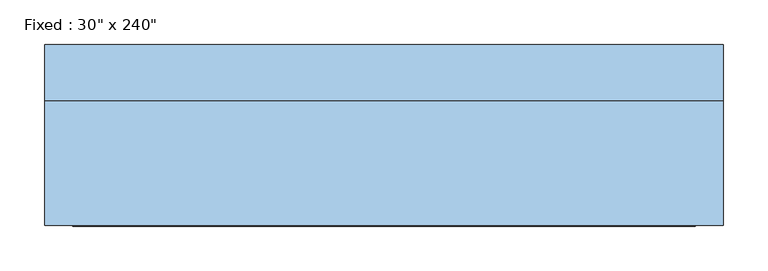
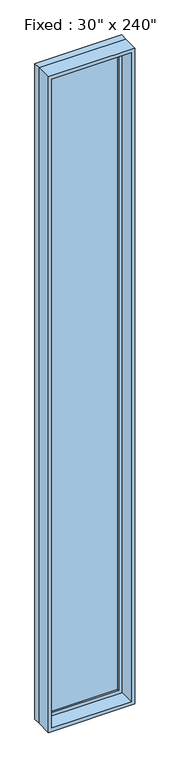
"""IFC4 building model written with IfcOpenShell, lengths in millimetres: window geometry."""

from ifc_helpers import new_model, si_unit, frame, origin, place, context, project, spatial, polyline, outline, extrude, source, transform, mapped, element, save


def window_1e0399d0(model_context):
    return source(origin(), model_context, "Body", "SweptSolid", [
        extrude(outline(polyline([(279.4, 53.975), (-355.6, 53.975), (-355.6, 66.675), (279.4, 66.675), (279.4, 53.975)])), frame((0.0, 0.0, 977.9), z_axis=(0.0, 0.0, 1.0), x_axis=(1.0, 0.0, 0.0)), (0.0, 0.0, 1.0), 5969.0),
        extrude(outline(polyline([(6991.35, -400.05), (933.45, -400.05), (933.45, 323.85), (6991.35, 323.85), (6991.35, -400.05)]), holes=[polyline([(6946.9, -355.6), (6946.9, 279.4), (977.9, 279.4), (977.9, -355.6), (6946.9, -355.6)])]), frame((0.0, 38.1, 0.0), z_axis=(0.0, 1.0, 0.0), x_axis=(0.0, 0.0, 1.0)), (0.0, 0.0, 1.0), 44.45),
        extrude(outline(polyline([(7010.4, -419.1), (914.4, -419.1), (914.4, 342.9), (7010.4, 342.9), (7010.4, -419.1)]), holes=[polyline([(6978.65, -387.35), (6978.65, 311.15), (946.15, 311.15), (946.15, -387.35), (6978.65, -387.35)])]), frame((0.0, -101.6, 0.0), z_axis=(0.0, 1.0, 0.0), x_axis=(0.0, 0.0, 1.0)), (0.0, 0.0, 1.0), 139.7),
        extrude(outline(polyline([(7010.4, 342.9), (7010.4, -419.1), (914.4, -419.1), (914.4, 342.9), (7010.4, 342.9)]), holes=[polyline([(6991.35, 323.85), (933.45, 323.85), (933.45, -400.05), (6991.35, -400.05), (6991.35, 323.85)])]), frame((0.0, 38.1, 0.0), z_axis=(0.0, 1.0, 0.0), x_axis=(0.0, 0.0, 1.0)), (0.0, 0.0, 1.0), 63.5),
    ])


if __name__ == "__main__":
    model = new_model("IFC4")
    model_context = context("Model", 3, world=origin())
    ifc_project = project(units=[si_unit("LENGTHUNIT", "METRE", prefix="MILLI")], contexts=[model_context])
    site = spatial("IfcSite", under=ifc_project)
    building = spatial("IfcBuilding", under=site)
    placement = place(None, origin())
    window_shape = window_1e0399d0(model_context)
    element("IfcWindow", 1, ObjectType="Fixed : 30\" x 240\"", at=placement, inside=building, context=model_context, shape_type="MappedRepresentation", body=[
        mapped(window_shape, transform((0.0, 0.0, 0.0), x_axis=(1.0, 0.0, 0.0), y_axis=(0.0, 1.0, 0.0), z_axis=(0.0, 0.0, 1.0))),
    ])
    save(model, "model.ifc")

# Revit data of these elements
# Type "Fixed : 30\" x 240\""
#   Type Mark = "21"
#   Construction Type Id = "GSP4R"
#   Assembly Code = "B2020100"
#   Analytic Construction = "1/8 in Pilkington single glazing"
#   Visual Light Transmittance = 0.9
#   Solar Heat Gain Coefficient = 0.78
#   Heat Transfer Coefficient (U) = 0.6496 BTU/(h·ft²·°F)
#   Height = 20' - 0"
#   Default Sill Height = 3' - 0"
#   Width = 2' - 6"
#   Window Inset = 0' - 0 3/4"
#   Define Thermal Properties by = 1
#   Glass Pane Material = Glass
#   Sash Material = Damp-proofing
#   Wall Closure = (empty or 0)
# Element 1 (IfcWindow, "Fixed : 30\" x 240\"")
#   Materials on its faces: "Damp-proofing", "Glass"
# Materials
#   "Glass": class "Glass", colour RGB 0 128 192, transparency 0.75, Description = "Soda Lime Glass", Cost = 0
#   "Damp-proofing": class "Generic", colour RGB 17 17 17, transparency 0, Description = "Damp-proofing", Cost = 0
